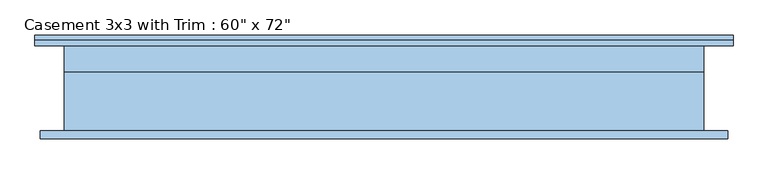
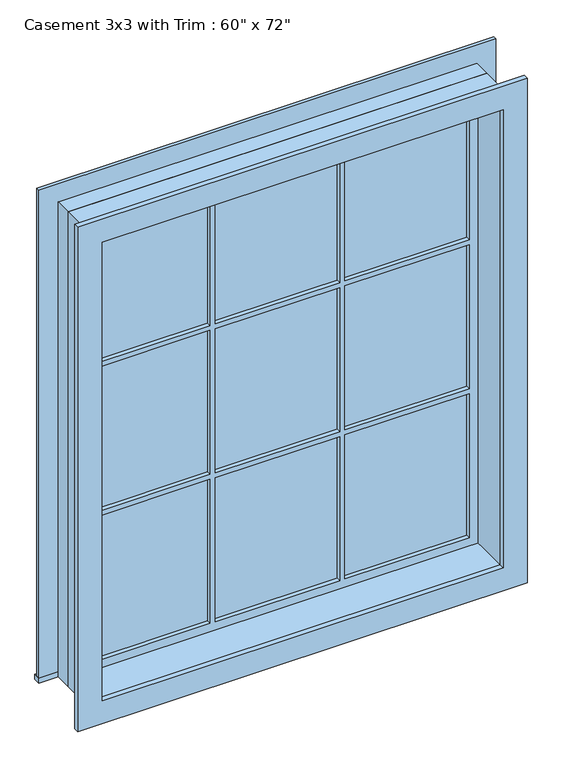
"""IFC4 building model written with IfcOpenShell, lengths in millimetres: window geometry."""

from ifc_helpers import new_model, si_unit, frame, origin, place, context, project, spatial, polyline, outline, extrude, source, transform, mapped, element, save


def window_f2d3b6b9(model_context):
    return source(origin(), model_context, "Body", "SweptSolid", [
        extrude(outline(polyline([(-831.85, 127.0), (831.85, 127.0), (831.85, 101.6), (-831.85, 101.6), (-831.85, 127.0)])), frame((0.0, 0.0, 914.4), z_axis=(0.0, 0.0, 1.0), x_axis=(1.0, 0.0, 0.0)), (0.0, 0.0, 1.0), 19.05),
        extrude(outline(polyline([(2724.15, -742.95), (2724.15, 742.95), (933.45, 742.95), (933.45, 831.85), (2813.05, 831.85), (2813.05, -831.85), (933.45, -831.85), (933.45, -742.95), (2724.15, -742.95)])), frame((0.0, 101.6, 0.0), z_axis=(0.0, 1.0, 0.0), x_axis=(0.0, 0.0, 1.0)), (0.0, 0.0, 1.0), 12.7),
        extrude(outline(polyline([(245.5333333, 66.675), (698.5, 66.675), (698.5, 53.975), (245.5333333, 53.975), (245.5333333, 66.675)])), frame((0.0, 0.0, 2125.1333333), z_axis=(0.0, 0.0, 1.0), x_axis=(1.0, 0.0, 0.0)), (0.0, 0.0, 1.0), 554.5666667),
        extrude(outline(polyline([(-226.4833333, 66.675), (226.4833333, 66.675), (226.4833333, 53.975), (-226.4833333, 53.975), (-226.4833333, 66.675)])), frame((0.0, 0.0, 2125.1333333), z_axis=(0.0, 0.0, 1.0), x_axis=(1.0, 0.0, 0.0)), (0.0, 0.0, 1.0), 554.5666667),
        extrude(outline(polyline([(-698.5, 66.675), (-245.5333333, 66.675), (-245.5333333, 53.975), (-698.5, 53.975), (-698.5, 66.675)])), frame((0.0, 0.0, 2125.1333333), z_axis=(0.0, 0.0, 1.0), x_axis=(1.0, 0.0, 0.0)), (0.0, 0.0, 1.0), 554.5666667),
        extrude(outline(polyline([(-698.5, 66.675), (-245.5333333, 66.675), (-245.5333333, 53.975), (-698.5, 53.975), (-698.5, 66.675)])), frame((0.0, 0.0, 1551.5166667), z_axis=(0.0, 0.0, 1.0), x_axis=(1.0, 0.0, 0.0)), (0.0, 0.0, 1.0), 554.5666667),
        extrude(outline(polyline([(-226.4833333, 66.675), (226.4833333, 66.675), (226.4833333, 53.975), (-226.4833333, 53.975), (-226.4833333, 66.675)])), frame((0.0, 0.0, 1551.5166667), z_axis=(0.0, 0.0, 1.0), x_axis=(1.0, 0.0, 0.0)), (0.0, 0.0, 1.0), 554.5666667),
        extrude(outline(polyline([(245.5333333, 66.675), (698.5, 66.675), (698.5, 53.975), (245.5333333, 53.975), (245.5333333, 66.675)])), frame((0.0, 0.0, 1551.5166667), z_axis=(0.0, 0.0, 1.0), x_axis=(1.0, 0.0, 0.0)), (0.0, 0.0, 1.0), 554.5666667),
        extrude(outline(polyline([(245.5333333, 66.675), (698.5, 66.675), (698.5, 53.975), (245.5333333, 53.975), (245.5333333, 66.675)])), frame((0.0, 0.0, 977.9), z_axis=(0.0, 0.0, 1.0), x_axis=(1.0, 0.0, 0.0)), (0.0, 0.0, 1.0), 554.5666667),
        extrude(outline(polyline([(-226.4833333, 66.675), (226.4833333, 66.675), (226.4833333, 53.975), (-226.4833333, 53.975), (-226.4833333, 66.675)])), frame((0.0, 0.0, 977.9), z_axis=(0.0, 0.0, 1.0), x_axis=(1.0, 0.0, 0.0)), (0.0, 0.0, 1.0), 554.5666667),
        extrude(outline(polyline([(-698.5, 66.675), (-245.5333333, 66.675), (-245.5333333, 53.975), (-698.5, 53.975), (-698.5, 66.675)])), frame((0.0, 0.0, 977.9), z_axis=(0.0, 0.0, 1.0), x_axis=(1.0, 0.0, 0.0)), (0.0, 0.0, 1.0), 554.5666667),
        extrude(outline(polyline([(2800.35, 819.15), (2800.35, -819.15), (857.25, -819.15), (857.25, 819.15), (2800.35, 819.15)]), holes=[polyline([(2711.45, 730.25), (946.15, 730.25), (946.15, -730.25), (2711.45, -730.25), (2711.45, 730.25)])]), frame((0.0, -120.65, 0.0), z_axis=(0.0, 1.0, 0.0), x_axis=(0.0, 0.0, 1.0)), (0.0, 0.0, 1.0), 19.05),
        extrude(outline(polyline([(2724.15, -742.95), (933.45, -742.95), (933.45, 742.95), (2724.15, 742.95), (2724.15, -742.95)]), holes=[polyline([(2679.7, -245.5333333), (2125.1333333, -245.5333333), (2125.1333333, -698.5), (2679.7, -698.5), (2679.7, -245.5333333)]), polyline([(2106.0833333, -245.5333333), (1551.5166667, -245.5333333), (1551.5166667, -698.5), (2106.0833333, -698.5), (2106.0833333, -245.5333333)]), polyline([(1532.4666667, -245.5333333), (977.9, -245.5333333), (977.9, -698.5), (1532.4666667, -698.5), (1532.4666667, -245.5333333)]), polyline([(2679.7, 226.4833333), (2125.1333333, 226.4833333), (2125.1333333, -226.4833333), (2679.7, -226.4833333), (2679.7, 226.4833333)]), polyline([(2106.0833333, 226.4833333), (1551.5166667, 226.4833333), (1551.5166667, -226.4833333), (2106.0833333, -226.4833333), (2106.0833333, 226.4833333)]), polyline([(1532.4666667, 226.4833333), (977.9, 226.4833333), (977.9, -226.4833333), (1532.4666667, -226.4833333), (1532.4666667, 226.4833333)]), polyline([(2679.7, 698.5), (2125.1333333, 698.5), (2125.1333333, 245.5333333), (2679.7, 245.5333333), (2679.7, 698.5)]), polyline([(2106.0833333, 698.5), (1551.5166667, 698.5), (1551.5166667, 245.5333333), (2106.0833333, 245.5333333), (2106.0833333, 698.5)]), polyline([(1532.4666667, 698.5), (977.9, 698.5), (977.9, 245.5333333), (1532.4666667, 245.5333333), (1532.4666667, 698.5)])]), frame((0.0, 38.1, 0.0), z_axis=(0.0, 1.0, 0.0), x_axis=(0.0, 0.0, 1.0)), (0.0, 0.0, 1.0), 44.45),
        extrude(outline(polyline([(2743.2, -762.0), (914.4, -762.0), (914.4, 762.0), (2743.2, 762.0), (2743.2, -762.0)]), holes=[polyline([(2711.45, -730.25), (2711.45, 730.25), (946.15, 730.25), (946.15, -730.25), (2711.45, -730.25)])]), frame((0.0, -101.6, 0.0), z_axis=(0.0, 1.0, 0.0), x_axis=(0.0, 0.0, 1.0)), (0.0, 0.0, 1.0), 139.7),
        extrude(outline(polyline([(2743.2, 762.0), (2743.2, -762.0), (914.4, -762.0), (914.4, 762.0), (2743.2, 762.0)]), holes=[polyline([(2724.15, 742.95), (933.45, 742.95), (933.45, -742.95), (2724.15, -742.95), (2724.15, 742.95)])]), frame((0.0, 38.1, 0.0), z_axis=(0.0, 1.0, 0.0), x_axis=(0.0, 0.0, 1.0)), (0.0, 0.0, 1.0), 63.5),
    ])


if __name__ == "__main__":
    model = new_model("IFC4")
    model_context = context("Model", 3, world=origin())
    ifc_project = project(units=[si_unit("LENGTHUNIT", "METRE", prefix="MILLI")], contexts=[model_context])
    site = spatial("IfcSite", under=ifc_project)
    building = spatial("IfcBuilding", under=site)
    placement = place(None, origin())
    window_shape = window_f2d3b6b9(model_context)
    element("IfcWindow", 1, ObjectType="Casement 3x3 with Trim : 60\" x 72\"", at=placement, inside=building, context=model_context, shape_type="MappedRepresentation", body=[
        mapped(window_shape, transform((0.0, 0.0, 0.0), x_axis=(1.0, 0.0, 0.0), y_axis=(0.0, 1.0, 0.0), z_axis=(0.0, 0.0, 1.0))),
    ])
    save(model, "model.ifc")

# Revit data of these elements
# Type "Casement 3x3 with Trim : 60\" x 72\""
#   Type Mark = "10"
#   Construction Type Id = "GSP4R"
#   Assembly Code = "B2020100"
#   Analytic Construction = "1/8 in Pilkington single glazing"
#   Visual Light Transmittance = 0.9
#   Solar Heat Gain Coefficient = 0.78
#   Heat Transfer Coefficient (U) = 0.6496 BTU/(h·ft²·°F)
#   Height = 6' - 0"
#   Default Sill Height = 3' - 0"
#   Trim Projection - Ext. = 0' - 0 1/2"
#   Trim Projection - Int. = 0' - 0 3/4"
#   Trim Width - Exterior = 0' - 3 1/2"
#   Trim Width - Interior = 0' - 3 1/2"
#   Width = 5' - 0"
#   Window Inset = 0' - 0 3/4"
#   Define Thermal Properties by = 1
#   Glass Pane Material = Glass
#   Sash Material = Sash
#   Trim Exterior Material = Trim
#   Trim Interior Material = Trim
#   Wall Closure = (empty or 0)
# Element 1 (IfcWindow, "Casement 3x3 with Trim : 60\" x 72\"")
#   Materials on its faces: "Sash", "Glass", "Trim"
# Materials
#   "Glass": class "Glass", colour RGB 0 128 192, transparency 0.75, Description = "Soda Lime Glass", Cost = 0
#   "Sash": class "Wood", colour RGB 224 178 126, transparency 0
#   "Trim": class "Wood", colour RGB 224 178 126, transparency 0
